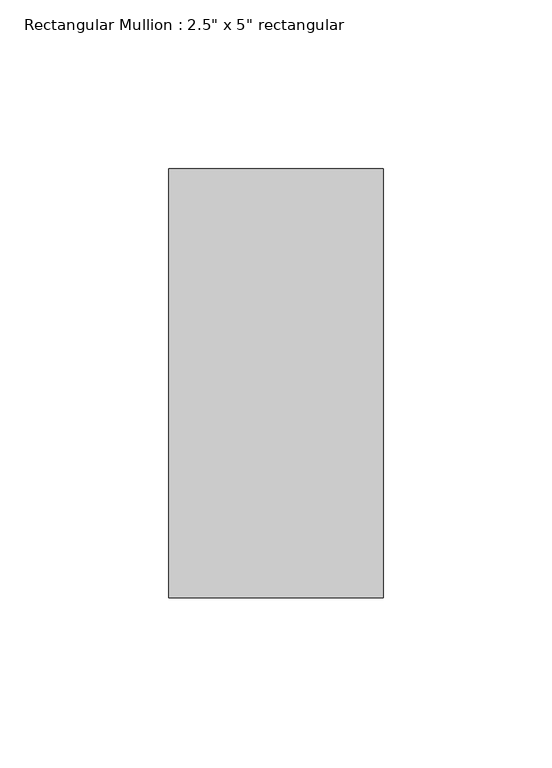
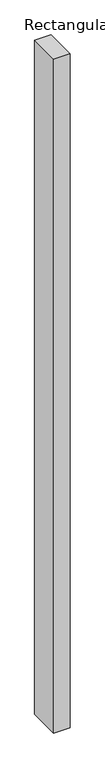
"""IFC4 building model written with IfcOpenShell, lengths in millimetres: member geometry."""

from ifc_helpers import new_model, si_unit, frame, origin, place, context, project, spatial, polyline, outline, extrude, source, transform, mapped, element, save


def member_923d5781(model_context):
    return source(origin(), model_context, "Body", "SweptSolid", [
        extrude(outline(polyline([(31.75, 63.5), (31.75, -63.5), (-31.75, -63.5), (-31.75, 63.5), (31.75, 63.5)])), frame((0.0, 0.0, -2743.2), z_axis=(0.0, 0.0, 1.0), x_axis=(1.0, 0.0, 0.0)), (0.0, 0.0, 1.0), 2743.2),
    ])


if __name__ == "__main__":
    model = new_model("IFC4")
    model_context = context("Model", 3, world=origin())
    ifc_project = project(units=[si_unit("LENGTHUNIT", "METRE", prefix="MILLI")], contexts=[model_context])
    site = spatial("IfcSite", under=ifc_project)
    building = spatial("IfcBuilding", under=site)
    placement = place(None, origin())
    member_shape = member_923d5781(model_context)
    element("IfcMember", 1, ObjectType="Rectangular Mullion : 2.5\" x 5\" rectangular", at=placement, inside=building, context=model_context, shape_type="MappedRepresentation", body=[
        mapped(member_shape, transform((0.0, 0.0, 0.0), x_axis=(1.0, 0.0, 0.0), y_axis=(0.0, 1.0, 0.0), z_axis=(0.0, 0.0, 1.0))),
    ])
    save(model, "model.ifc")

# Revit data of these elements
# Type "Rectangular Mullion : 2.5\" x 5\" rectangular"
#   built-in parameter 1007304 = 0.416667 (stored number, unit not read)
#   built-in parameter 1007301 = 0.104167 (stored number, unit not read)
#   built-in parameter 1007300 = 0.104167 (stored number, unit not read)
# Element 1 (IfcMember, "Rectangular Mullion : 2.5\" x 5\" rectangular")
#   Materials on its faces: "Aluminum"
# Materials
#   "Aluminum": class "Metal", colour RGB 247 247 247, transparency 0, Description = "Aluminum 6061", Cost = 0
